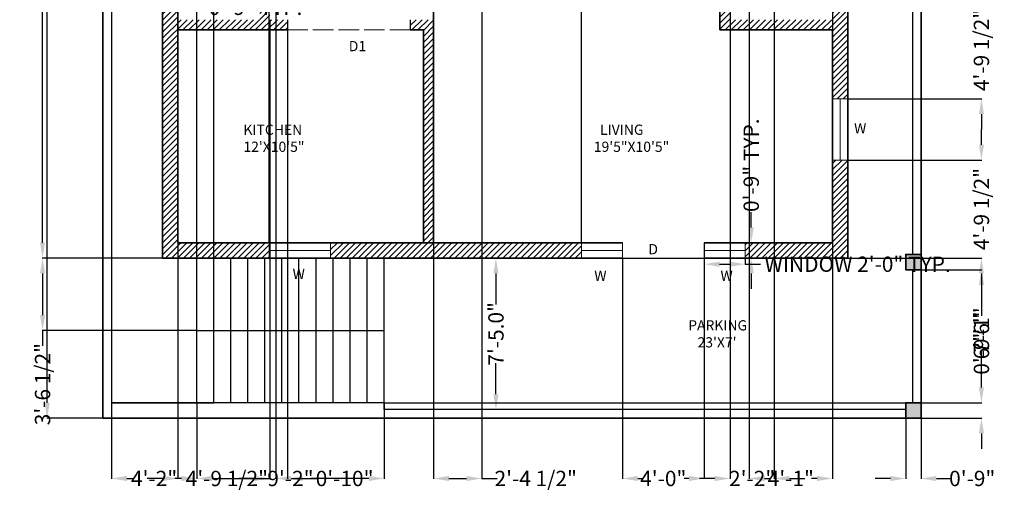
# Model space of a CAD drawing. Units: inches. Extents: x 287 to 864, y 208 to 990.
# Tile 1 of 3: x 287 to 864, y 208 to 491. Entities that reach past the tile are written whole.
import ezdxf

# ---------------------------------------------------------------- set-up
doc = ezdxf.new("R2010")
doc.units = ezdxf.units.IN
doc.header["$MEASUREMENT"] = 0
doc.linetypes.add('ACAD_ISO02W100', pattern=[15, 12, -3])
for name, color, linetype, lineweight in [('A-ANNO-DIMS', 2, 'Continuous', 18), ('A-ANNO-TEXT', 7, 'Continuous', 18), ('A-AREA-IDEN', 7, 'Continuous', 18), ('A-COLS', 7, 'Continuous', 35), ('A-DOOR', 3, 'Continuous', 25), ('A-FLOR-STRS', 7, 'Continuous', 25), ('A-GLAZ', 4, 'Continuous', 18), ('A-SITE-WALL', 7, 'Continuous', 30), ('A-WALL', 7, 'Continuous', 35), ('A-WALL-OVHD', 7, 'ACAD_ISO02W100', 18), ('C-PROP', 7, 'Continuous', 35)]:
    doc.layers.add(name, color=color, linetype=linetype, lineweight=lineweight)
doc.layers.add('A-COLS-PATT', color=18, linetype='Continuous', lineweight=13, true_color=0x000000)
doc.layers.add('A-WALL-PATT', color=240, linetype='Continuous', lineweight=13, true_color=0xed1f24)
doc.styles.get("Standard").update_dxf_attribs({"font": 'arial.ttf'})
doc.dimstyles.get("Standard").update_dxf_attribs({"dimtxt": 9, "dimasz": 9, "dimexe": 0.18, "dimexo": 0.0625, "dimgap": 0.09, "dimtad": 0, "dimdec": 1, "dimzin": 0, "dimdsep": 46, "dimlunit": 3, "dimtxsty": 'Standard', "dimcen": 0.09, "dimadec": 0, "dimazin": 0, "dimtfac": 1, "dimtdec": 1, "dimtofl": 0, "dimtmove": 0, "dimatfit": 3, "dimfxl": 1, "dimtolj": 1, "dimtzin": 0, "dimarcsym": 0})

# ---------------------------------------------------------------- blocks, each defined once
blk = doc.blocks.new('*D2')
at = {"layer": 'A-ANNO-DIMS', "color": 0, "lineweight": -2, "transparency": 16777216}
for p, q in [((335.53, 941.05), (302.65, 941.05)), ((302.83, 932.05), (302.83, 606.78)), ((302.83, 266.05), (302.83, 591.33)), ((335.53, 257.05), (302.65, 257.05))]:
    blk.add_line(p, q, dxfattribs=at)
at = {"layer": 'A-ANNO-DIMS', "color": 0, "transparency": 16777216}
for points in [[(301.33, 932.05), (304.33, 932.05), (302.83, 941.05)], [(301.33, 266.05), (304.33, 266.05), (302.83, 257.05)]]:
    blk.add_solid(points, dxfattribs=at)
at = {"layer": 'Defpoints', "color": 0, "transparency": 16777216}
for p in [(335.59, 941.05), (302.83, 257.05), (335.59, 257.05)]:
    blk.add_point(p, dxfattribs=at)
at = {"layer": 'A-ANNO-DIMS', "color": 0, "transparency": 16777216, "insert": (302.83, 599.05), "char_height": 9, "attachment_point": 5, "rotation": 90}
blk.add_mtext("\\A1;57'", dxfattribs=at)
blk = doc.blocks.new('*D5')
at = {"layer": 'A-ANNO-DIMS', "color": 0, "lineweight": -2, "transparency": 16777216}
for p, q in [((566.22, 351.05), (566.34, 351.05)), ((566.16, 342.05), (566.16, 323.81)), ((566.16, 271.05), (566.16, 289.3)), ((566.22, 262.05), (566.34, 262.05))]:
    blk.add_line(p, q, dxfattribs=at)
at = {"layer": 'A-ANNO-DIMS', "color": 0, "transparency": 16777216}
for points in [[(564.66, 342.05), (567.66, 342.05), (566.16, 351.05)], [(564.66, 271.05), (567.66, 271.05), (566.16, 262.05)]]:
    blk.add_solid(points, dxfattribs=at)
at = {"layer": 'Defpoints', "color": 0, "transparency": 16777216}
for p in [(566.16, 351.05), (566.16, 262.05), (566.16, 262.05)]:
    blk.add_point(p, dxfattribs=at)
at = {"layer": 'A-ANNO-DIMS', "color": 0, "transparency": 16777216, "insert": (566.16, 306.55), "char_height": 9, "attachment_point": 5, "rotation": 90}
blk.add_mtext('\\A1;7\'-5.0"', dxfattribs=at)
blk = doc.blocks.new('WIN-36IN')
for p, q in [((0, 9), (0, 0)), ((36, 9), (36, 0)), ((0, 4.5), (36, 4.5))]:
    blk.add_line(p, q)
blk = doc.blocks.new('WIN-24IN')
for p, q in [((0, 0), (0, 9)), ((24, 0), (24, 9)), ((24, 4.5), (0, 4.5))]:
    blk.add_line(p, q)
blk = doc.blocks.new('*D20')
at = {"layer": 'A-ANNO-DIMS', "color": 0, "lineweight": -2, "transparency": 16777216}
for p, q in [((361.59, 498.3), (352.59, 498.3)), ((370.59, 501.84), (370.59, 498.12)), ((379.59, 501.84), (379.59, 498.12)), ((388.59, 498.3), (397.59, 498.3))]:
    blk.add_line(p, q, dxfattribs=at)
at = {"layer": 'A-ANNO-DIMS', "color": 0, "transparency": 16777216}
for points in [[(361.59, 499.8), (361.59, 496.8), (370.59, 498.3)], [(388.59, 499.8), (388.59, 496.8), (379.59, 498.3)]]:
    blk.add_solid(points, dxfattribs=at)
at = {"layer": 'Defpoints', "color": 0, "transparency": 16777216}
for p in [(370.59, 501.9), (379.59, 501.9), (379.59, 498.3)]:
    blk.add_point(p, dxfattribs=at)
at = {"layer": 'A-ANNO-DIMS', "color": 0, "transparency": 16777216, "insert": (425.11, 498.3), "char_height": 9, "attachment_point": 5}
blk.add_mtext('\\A1;0\'-9" TYP.', dxfattribs=at)
blk = doc.blocks.new('*D21')
at = {"layer": 'A-ANNO-DIMS', "color": 0, "lineweight": -2, "transparency": 16777216}
for p, q in [((688.36, 350.99), (688.36, 347.27)), ((697.36, 347.45), (703.36, 347.45)), ((712.36, 350.99), (712.36, 347.27)), ((712.36, 347.45), (721.36, 347.45))]:
    blk.add_line(p, q, dxfattribs=at)
at = {"layer": 'A-ANNO-DIMS', "color": 0, "transparency": 16777216}
for points in [[(697.36, 348.95), (697.36, 345.95), (688.36, 347.45)], [(703.36, 348.95), (703.36, 345.95), (712.36, 347.45)]]:
    blk.add_solid(points, dxfattribs=at)
at = {"layer": 'Defpoints', "color": 0, "transparency": 16777216}
for p in [(688.36, 351.05), (712.36, 351.05), (712.36, 347.45)]:
    blk.add_point(p, dxfattribs=at)
at = {"layer": 'A-ANNO-DIMS', "color": 0, "transparency": 16777216, "insert": (778.39, 347.45), "char_height": 9, "attachment_point": 5}
blk.add_mtext('\\A1;WINDOW 2\'-0" TYP.', dxfattribs=at)
blk = doc.blocks.new('*D22')
at = {"layer": 'A-ANNO-DIMS', "color": 0, "lineweight": -2, "transparency": 16777216}
for p, q in [((715.96, 369.05), (715.96, 378.05)), ((712.42, 360.05), (716.14, 360.05)), ((712.42, 351.05), (716.14, 351.05)), ((715.96, 342.05), (715.96, 333.05))]:
    blk.add_line(p, q, dxfattribs=at)
at = {"layer": 'A-ANNO-DIMS', "color": 0, "transparency": 16777216}
for points in [[(714.46, 369.05), (717.46, 369.05), (715.96, 360.05)], [(714.46, 342.05), (717.46, 342.05), (715.96, 351.05)]]:
    blk.add_solid(points, dxfattribs=at)
at = {"layer": 'Defpoints', "color": 0, "transparency": 16777216}
for p in [(712.36, 360.05), (715.96, 360.05), (712.36, 351.05)]:
    blk.add_point(p, dxfattribs=at)
at = {"layer": 'A-ANNO-DIMS', "color": 0, "transparency": 16777216, "insert": (715.96, 405.57), "char_height": 9, "attachment_point": 5, "rotation": 90}
blk.add_mtext('\\A1;0\'-9" TYP.', dxfattribs=at)
blk = doc.blocks.new('*D24')
at = {"layer": 'A-ANNO-DIMS', "color": 0, "lineweight": -2, "transparency": 16777216}
for p, q in [((370.53, 906.05), (299.96, 906.05)), ((300.14, 897.05), (300.14, 644.28)), ((300.14, 360.05), (300.14, 612.83)), ((370.53, 351.05), (299.96, 351.05))]:
    blk.add_line(p, q, dxfattribs=at)
at = {"layer": 'A-ANNO-DIMS', "color": 0, "transparency": 16777216}
for points in [[(298.64, 897.05), (301.64, 897.05), (300.14, 906.05)], [(298.64, 360.05), (301.64, 360.05), (300.14, 351.05)]]:
    blk.add_solid(points, dxfattribs=at)
at = {"layer": 'Defpoints', "color": 0, "transparency": 16777216}
for p in [(300.14, 906.05), (370.59, 906.05), (370.59, 351.05)]:
    blk.add_point(p, dxfattribs=at)
at = {"layer": 'A-ANNO-DIMS', "color": 0, "transparency": 16777216, "insert": (300.14, 628.55), "char_height": 9, "attachment_point": 5, "rotation": 90}
blk.add_mtext('\\A1;46\'-3"', dxfattribs=at)
blk = doc.blocks.new('*D25')
at = {"layer": 'A-ANNO-DIMS', "color": 0, "lineweight": -2, "transparency": 16777216}
for p, q in [((390.59, 265.99), (390.59, 221.42)), ((500.59, 265.99), (500.59, 221.42)), ((399.59, 221.6), (433.54, 221.6)), ((491.59, 221.6), (457.64, 221.6))]:
    blk.add_line(p, q, dxfattribs=at)
at = {"layer": 'A-ANNO-DIMS', "color": 0, "transparency": 16777216}
for points in [[(399.59, 223.1), (399.59, 220.1), (390.59, 221.6)], [(491.59, 223.1), (491.59, 220.1), (500.59, 221.6)]]:
    blk.add_solid(points, dxfattribs=at)
at = {"layer": 'Defpoints', "color": 0, "transparency": 16777216}
for p in [(390.59, 266.05), (500.59, 266.05), (500.59, 221.6)]:
    blk.add_point(p, dxfattribs=at)
at = {"layer": 'A-ANNO-DIMS', "color": 0, "transparency": 16777216, "insert": (445.59, 221.6), "char_height": 9, "attachment_point": 5}
blk.add_mtext('\\A1;9\'-2"', dxfattribs=at)
blk = doc.blocks.new('*D26')
at = {"layer": 'A-ANNO-DIMS', "color": 0, "lineweight": -2, "transparency": 16777216}
for p, q in [((390.53, 351.05), (299.96, 351.05)), ((300.14, 342.05), (300.14, 317.55)), ((390.53, 308.55), (299.96, 308.55)), ((300.14, 308.55), (300.14, 299.55))]:
    blk.add_line(p, q, dxfattribs=at)
at = {"layer": 'A-ANNO-DIMS', "color": 0, "transparency": 16777216}
for points in [[(298.64, 342.05), (301.64, 342.05), (300.14, 351.05)], [(298.64, 317.55), (301.64, 317.55), (300.14, 308.55)]]:
    blk.add_solid(points, dxfattribs=at)
at = {"layer": 'Defpoints', "color": 0, "transparency": 16777216}
for p in [(390.59, 351.05), (300.14, 308.55), (390.59, 308.55)]:
    blk.add_point(p, dxfattribs=at)
at = {"layer": 'A-ANNO-DIMS', "color": 0, "transparency": 16777216, "insert": (300.14, 277.02), "char_height": 9, "attachment_point": 5, "rotation": 90}
blk.add_mtext('\\A1;3\'-6 1/2"', dxfattribs=at)
blk = doc.blocks.new('*D27')
at = {"layer": 'A-ANNO-DIMS', "color": 0, "lineweight": -2, "transparency": 16777216}
for p, q in [((500.65, 351.05), (851.22, 351.05)), ((851.04, 342.05), (851.04, 320.57)), ((851.04, 275.05), (851.04, 296.54)), ((500.65, 266.05), (851.22, 266.05))]:
    blk.add_line(p, q, dxfattribs=at)
at = {"layer": 'A-ANNO-DIMS', "color": 0, "transparency": 16777216}
for points in [[(849.54, 342.05), (852.54, 342.05), (851.04, 351.05)], [(849.54, 275.05), (852.54, 275.05), (851.04, 266.05)]]:
    blk.add_solid(points, dxfattribs=at)
at = {"layer": 'Defpoints', "color": 0, "transparency": 16777216}
for p in [(500.59, 351.05), (500.59, 266.05), (851.04, 266.05)]:
    blk.add_point(p, dxfattribs=at)
at = {"layer": 'A-ANNO-DIMS', "color": 0, "transparency": 16777216, "insert": (851.04, 308.55), "char_height": 9, "attachment_point": 5, "rotation": 90}
blk.add_mtext('\\A1;7\'-1"', dxfattribs=at)
blk = doc.blocks.new('*D28')
at = {"layer": 'A-ANNO-DIMS', "color": 0, "lineweight": -2, "transparency": 16777216}
for p, q in [((381.59, 976.5), (372.59, 976.5)), ((390.59, 351.12), (390.59, 976.68)), ((400.59, 351.12), (400.59, 976.68)), ((409.59, 976.5), (418.59, 976.5))]:
    blk.add_line(p, q, dxfattribs=at)
at = {"layer": 'A-ANNO-DIMS', "color": 0, "transparency": 16777216}
for points in [[(381.59, 978), (381.59, 975), (390.59, 976.5)], [(409.59, 978), (409.59, 975), (400.59, 976.5)]]:
    blk.add_solid(points, dxfattribs=at)
at = {"layer": 'Defpoints', "color": 0, "transparency": 16777216}
for p in [(400.59, 976.5), (390.59, 351.05), (400.59, 351.05)]:
    blk.add_point(p, dxfattribs=at)
at = {"layer": 'A-ANNO-DIMS', "color": 0, "transparency": 16777216, "insert": (434.14, 976.5), "char_height": 9, "attachment_point": 5}
blk.add_mtext('\\A1;0\'-10"', dxfattribs=at)
blk = doc.blocks.new('*D29')
at = {"layer": 'A-ANNO-DIMS', "color": 0, "lineweight": -2, "transparency": 16777216}
for p, q in [((340.59, 265.99), (340.59, 221.42)), ((390.59, 265.99), (390.59, 221.42)), ((349.59, 221.6), (353.36, 221.6)), ((381.59, 221.6), (377.82, 221.6))]:
    blk.add_line(p, q, dxfattribs=at)
at = {"layer": 'A-ANNO-DIMS', "color": 0, "transparency": 16777216}
for points in [[(349.59, 223.1), (349.59, 220.1), (340.59, 221.6)], [(381.59, 223.1), (381.59, 220.1), (390.59, 221.6)]]:
    blk.add_solid(points, dxfattribs=at)
at = {"layer": 'Defpoints', "color": 0, "transparency": 16777216}
for p in [(340.59, 266.05), (390.59, 266.05), (390.59, 221.6)]:
    blk.add_point(p, dxfattribs=at)
at = {"layer": 'A-ANNO-DIMS', "color": 0, "transparency": 16777216, "insert": (365.59, 221.6), "char_height": 9, "attachment_point": 5}
blk.add_mtext('\\A1;4\'-2"', dxfattribs=at)
blk = doc.blocks.new('*D30')
at = {"layer": 'A-ANNO-DIMS', "color": 0, "lineweight": -2, "transparency": 16777216}
for p, q in [((640.36, 350.99), (640.36, 221.42)), ((688.36, 350.99), (688.36, 221.42)), ((649.36, 221.6), (652.13, 221.6)), ((679.36, 221.6), (676.59, 221.6))]:
    blk.add_line(p, q, dxfattribs=at)
at = {"layer": 'A-ANNO-DIMS', "color": 0, "transparency": 16777216}
for points in [[(649.36, 223.1), (649.36, 220.1), (640.36, 221.6)], [(679.36, 223.1), (679.36, 220.1), (688.36, 221.6)]]:
    blk.add_solid(points, dxfattribs=at)
at = {"layer": 'Defpoints', "color": 0, "transparency": 16777216}
for p in [(640.36, 351.05), (688.36, 351.05), (688.36, 221.6)]:
    blk.add_point(p, dxfattribs=at)
at = {"layer": 'A-ANNO-DIMS', "color": 0, "transparency": 16777216, "insert": (664.36, 221.6), "char_height": 9, "attachment_point": 5}
blk.add_mtext('\\A1;4\'-0"', dxfattribs=at)
blk = doc.blocks.new('*D32')
at = {"layer": 'A-ANNO-DIMS', "color": 0, "lineweight": -2, "transparency": 16777216}
for p, q in [((433.59, 490.99), (433.59, 221.42)), ((443.82, 484.99), (443.82, 221.42)), ((424.59, 221.6), (415.59, 221.6)), ((452.82, 221.6), (461.82, 221.6))]:
    blk.add_line(p, q, dxfattribs=at)
at = {"layer": 'A-ANNO-DIMS', "color": 0, "transparency": 16777216}
for points in [[(424.59, 223.1), (424.59, 220.1), (433.59, 221.6)], [(452.82, 223.1), (452.82, 220.1), (443.82, 221.6)]]:
    blk.add_solid(points, dxfattribs=at)
at = {"layer": 'Defpoints', "color": 0, "transparency": 16777216}
for p in [(433.59, 491.05), (443.82, 485.05), (443.82, 221.6)]:
    blk.add_point(p, dxfattribs=at)
at = {"layer": 'A-ANNO-DIMS', "color": 0, "transparency": 16777216, "insert": (477.37, 221.6), "char_height": 9, "attachment_point": 5}
blk.add_mtext('\\A1;0\'-10"', dxfattribs=at)
blk = doc.blocks.new('*D33')
at = {"layer": 'A-ANNO-DIMS', "color": 0, "lineweight": -2, "transparency": 16777216}
for p, q in [((379.59, 896.99), (379.59, 221.42)), ((436.99, 896.99), (436.99, 221.42)), ((370.59, 221.6), (361.59, 221.6)), ((445.99, 221.6), (454.99, 221.6))]:
    blk.add_line(p, q, dxfattribs=at)
at = {"layer": 'A-ANNO-DIMS', "color": 0, "transparency": 16777216}
for points in [[(370.59, 223.1), (370.59, 220.1), (379.59, 221.6)], [(445.99, 223.1), (445.99, 220.1), (436.99, 221.6)]]:
    blk.add_solid(points, dxfattribs=at)
at = {"layer": 'Defpoints', "color": 0, "transparency": 16777216}
for p in [(379.59, 897.05), (436.99, 897.05), (436.99, 221.6)]:
    blk.add_point(p, dxfattribs=at)
at = {"layer": 'A-ANNO-DIMS', "color": 0, "transparency": 16777216, "insert": (408.29, 221.6), "char_height": 9, "attachment_point": 5}
blk.add_mtext('\\A1;4\'-9 1/2"', dxfattribs=at)
blk = doc.blocks.new('*D34')
at = {"layer": 'A-ANNO-DIMS', "color": 0, "lineweight": -2, "transparency": 16777216}
for p, q in [((529.59, 896.99), (529.59, 221.42)), ((557.92, 896.99), (557.92, 221.42)), ((538.59, 221.6), (548.92, 221.6)), ((557.92, 221.6), (566.92, 221.6))]:
    blk.add_line(p, q, dxfattribs=at)
at = {"layer": 'A-ANNO-DIMS', "color": 0, "transparency": 16777216}
for points in [[(538.59, 223.1), (538.59, 220.1), (529.59, 221.6)], [(548.92, 223.1), (548.92, 220.1), (557.92, 221.6)]]:
    blk.add_solid(points, dxfattribs=at)
at = {"layer": 'Defpoints', "color": 0, "transparency": 16777216}
for p in [(529.59, 897.05), (557.92, 897.05), (557.92, 221.6)]:
    blk.add_point(p, dxfattribs=at)
at = {"layer": 'A-ANNO-DIMS', "color": 0, "transparency": 16777216, "insert": (589.53, 221.6), "char_height": 9, "attachment_point": 5}
blk.add_mtext('\\A1;2\'-4 1/2"', dxfattribs=at)
blk = doc.blocks.new('*D35')
at = {"layer": 'A-ANNO-DIMS', "color": 0, "lineweight": -2, "transparency": 16777216}
for p, q in [((714.78, 896.99), (714.78, 221.42)), ((763.59, 896.99), (763.59, 221.42)), ((723.78, 221.6), (726.95, 221.6)), ((754.59, 221.6), (751.42, 221.6))]:
    blk.add_line(p, q, dxfattribs=at)
at = {"layer": 'A-ANNO-DIMS', "color": 0, "transparency": 16777216}
for points in [[(723.78, 223.1), (723.78, 220.1), (714.78, 221.6)], [(754.59, 223.1), (754.59, 220.1), (763.59, 221.6)]]:
    blk.add_solid(points, dxfattribs=at)
at = {"layer": 'Defpoints', "color": 0, "transparency": 16777216}
for p in [(714.78, 897.05), (763.59, 897.05), (763.59, 221.6)]:
    blk.add_point(p, dxfattribs=at)
at = {"layer": 'A-ANNO-DIMS', "color": 0, "transparency": 16777216, "insert": (739.19, 221.6), "char_height": 9, "attachment_point": 5}
blk.add_mtext('\\A1;4\'-1"', dxfattribs=at)
blk = doc.blocks.new('*D37')
at = {"layer": 'A-ANNO-DIMS', "color": 0, "lineweight": -2, "transparency": 16777216}
for p, q in [((851.04, 510.9), (851.04, 519.9)), ((772.65, 501.9), (851.22, 501.9)), ((772.65, 444.61), (851.22, 444.61)), ((851.04, 435.61), (851.04, 426.61))]:
    blk.add_line(p, q, dxfattribs=at)
at = {"layer": 'A-ANNO-DIMS', "color": 0, "transparency": 16777216}
for points in [[(849.54, 510.9), (852.54, 510.9), (851.04, 501.9)], [(849.54, 435.61), (852.54, 435.61), (851.04, 444.61)]]:
    blk.add_solid(points, dxfattribs=at)
at = {"layer": 'Defpoints', "color": 0, "transparency": 16777216}
for p in [(772.59, 501.9), (851.04, 501.9), (772.59, 444.61)]:
    blk.add_point(p, dxfattribs=at)
at = {"layer": 'A-ANNO-DIMS', "color": 0, "transparency": 16777216, "insert": (851.04, 473.26), "char_height": 9, "attachment_point": 5, "rotation": 90}
blk.add_mtext('\\A1;4\'-9 1/2"', dxfattribs=at)
blk = doc.blocks.new('*D38')
at = {"layer": 'A-ANNO-DIMS', "color": 0, "lineweight": -2, "transparency": 16777216}
for p, q in [((851.04, 417.61), (851.04, 426.61)), ((772.65, 408.61), (851.22, 408.61)), ((772.65, 351.05), (851.22, 351.05)), ((851.04, 342.05), (851.04, 333.05))]:
    blk.add_line(p, q, dxfattribs=at)
at = {"layer": 'A-ANNO-DIMS', "color": 0, "transparency": 16777216}
for points in [[(849.54, 417.61), (852.54, 417.61), (851.04, 408.61)], [(849.54, 342.05), (852.54, 342.05), (851.04, 351.05)]]:
    blk.add_solid(points, dxfattribs=at)
at = {"layer": 'Defpoints', "color": 0, "transparency": 16777216}
for p in [(772.59, 408.61), (851.04, 408.61), (772.59, 351.05)]:
    blk.add_point(p, dxfattribs=at)
at = {"layer": 'A-ANNO-DIMS', "color": 0, "transparency": 16777216, "insert": (851.04, 379.83), "char_height": 9, "attachment_point": 5, "rotation": 90}
blk.add_mtext('\\A1;4\'-9 1/2"', dxfattribs=at)
blk = doc.blocks.new('*D39')
at = {"layer": 'A-ANNO-DIMS', "color": 0, "lineweight": -2, "transparency": 16777216}
for p, q in [((370.59, 976.5), (361.59, 976.5)), ((379.59, 360.12), (379.59, 976.68)), ((433.14, 360.12), (433.14, 976.68)), ((442.14, 976.5), (451.14, 976.5))]:
    blk.add_line(p, q, dxfattribs=at)
at = {"layer": 'A-ANNO-DIMS', "color": 0, "transparency": 16777216}
for points in [[(370.59, 978), (370.59, 975), (379.59, 976.5)], [(442.14, 978), (442.14, 975), (433.14, 976.5)]]:
    blk.add_solid(points, dxfattribs=at)
at = {"layer": 'Defpoints', "color": 0, "transparency": 16777216}
for p in [(433.14, 976.5), (379.59, 360.05), (433.14, 360.05)]:
    blk.add_point(p, dxfattribs=at)
at = {"layer": 'A-ANNO-DIMS', "color": 0, "transparency": 16777216, "insert": (406.37, 976.5), "char_height": 9, "attachment_point": 5}
blk.add_mtext('\\A1;4\'-5 1/2"', dxfattribs=at)
blk = doc.blocks.new('*D40')
at = {"layer": 'A-ANNO-DIMS', "color": 0, "lineweight": -2, "transparency": 16777216}
for p, q in [((529.59, 360.12), (529.59, 976.68)), ((538.59, 976.5), (560.96, 976.5)), ((607.36, 976.5), (584.99, 976.5)), ((616.36, 360.12), (616.36, 976.68))]:
    blk.add_line(p, q, dxfattribs=at)
at = {"layer": 'A-ANNO-DIMS', "color": 0, "transparency": 16777216}
for points in [[(538.59, 978), (538.59, 975), (529.59, 976.5)], [(607.36, 978), (607.36, 975), (616.36, 976.5)]]:
    blk.add_solid(points, dxfattribs=at)
at = {"layer": 'Defpoints', "color": 0, "transparency": 16777216}
for p in [(616.36, 976.5), (529.59, 360.05), (616.36, 360.05)]:
    blk.add_point(p, dxfattribs=at)
at = {"layer": 'A-ANNO-DIMS', "color": 0, "transparency": 16777216, "insert": (572.97, 976.5), "char_height": 9, "attachment_point": 5}
blk.add_mtext('\\A1;7\'-3"', dxfattribs=at)
blk = doc.blocks.new('*D47')
at = {"layer": 'A-ANNO-DIMS', "color": 0, "lineweight": -2, "transparency": 16777216}
for p, q in [((703.59, 584.99), (703.59, 221.42)), ((729.41, 584.99), (729.41, 221.42)), ((694.59, 221.6), (685.59, 221.6)), ((738.41, 221.6), (747.41, 221.6))]:
    blk.add_line(p, q, dxfattribs=at)
at = {"layer": 'A-ANNO-DIMS', "color": 0, "transparency": 16777216}
for points in [[(694.59, 223.1), (694.59, 220.1), (703.59, 221.6)], [(738.41, 223.1), (738.41, 220.1), (729.41, 221.6)]]:
    blk.add_solid(points, dxfattribs=at)
at = {"layer": 'Defpoints', "color": 0, "transparency": 16777216}
for p in [(703.59, 585.05), (729.41, 585.05), (729.41, 221.6)]:
    blk.add_point(p, dxfattribs=at)
at = {"layer": 'A-ANNO-DIMS', "color": 0, "transparency": 16777216, "insert": (716.5, 221.6), "char_height": 9, "attachment_point": 5}
blk.add_mtext('\\A1;2\'-2"', dxfattribs=at)
blk = doc.blocks.new('*D48')
at = {"layer": 'A-ANNO-DIMS', "color": 0, "lineweight": -2, "transparency": 16777216}
for p, q in [((815.65, 344.19), (851.22, 344.19)), ((851.04, 335.19), (851.04, 317.2)), ((851.04, 275.05), (851.04, 293.04)), ((815.65, 266.05), (851.22, 266.05))]:
    blk.add_line(p, q, dxfattribs=at)
at = {"layer": 'A-ANNO-DIMS', "color": 0, "transparency": 16777216}
for points in [[(849.54, 335.19), (852.54, 335.19), (851.04, 344.19)], [(849.54, 275.05), (852.54, 275.05), (851.04, 266.05)]]:
    blk.add_solid(points, dxfattribs=at)
at = {"layer": 'Defpoints', "color": 0, "transparency": 16777216}
for p in [(815.59, 344.19), (851.04, 344.19), (815.59, 266.05)]:
    blk.add_point(p, dxfattribs=at)
at = {"layer": 'A-ANNO-DIMS', "color": 0, "transparency": 16777216, "insert": (851.04, 305.12), "char_height": 9, "attachment_point": 5, "rotation": 90}
blk.add_mtext('\\A1;6\'-6"', dxfattribs=at)
blk = doc.blocks.new('*D49')
at = {"layer": 'A-ANNO-DIMS', "color": 0, "lineweight": -2, "transparency": 16777216}
for p, q in [((806.59, 256.99), (806.59, 221.42)), ((815.59, 256.99), (815.59, 221.42)), ((797.59, 221.6), (788.59, 221.6)), ((824.59, 221.6), (833.59, 221.6))]:
    blk.add_line(p, q, dxfattribs=at)
at = {"layer": 'A-ANNO-DIMS', "color": 0, "transparency": 16777216}
for points in [[(797.59, 223.1), (797.59, 220.1), (806.59, 221.6)], [(824.59, 223.1), (824.59, 220.1), (815.59, 221.6)]]:
    blk.add_solid(points, dxfattribs=at)
at = {"layer": 'Defpoints', "color": 0, "transparency": 16777216}
for p in [(806.59, 257.05), (815.59, 257.05), (815.59, 221.6)]:
    blk.add_point(p, dxfattribs=at)
at = {"layer": 'A-ANNO-DIMS', "color": 0, "transparency": 16777216, "insert": (845.64, 221.6), "char_height": 9, "attachment_point": 5}
blk.add_mtext('\\A1;0\'-9"', dxfattribs=at)
blk = doc.blocks.new('*D50')
at = {"layer": 'A-ANNO-DIMS', "color": 0, "lineweight": -2, "transparency": 16777216}
for p, q in [((851.04, 275.05), (851.04, 284.05)), ((815.65, 266.05), (851.22, 266.05)), ((815.65, 257.05), (851.22, 257.05)), ((851.04, 248.05), (851.04, 239.05))]:
    blk.add_line(p, q, dxfattribs=at)
at = {"layer": 'A-ANNO-DIMS', "color": 0, "transparency": 16777216}
for points in [[(849.54, 275.05), (852.54, 275.05), (851.04, 266.05)], [(849.54, 248.05), (852.54, 248.05), (851.04, 257.05)]]:
    blk.add_solid(points, dxfattribs=at)
at = {"layer": 'Defpoints', "color": 0, "transparency": 16777216}
for p in [(815.59, 266.05), (851.04, 266.05), (815.59, 257.05)]:
    blk.add_point(p, dxfattribs=at)
at = {"layer": 'A-ANNO-DIMS', "color": 0, "transparency": 16777216, "insert": (851.04, 296.11), "char_height": 9, "attachment_point": 5, "rotation": 90}
blk.add_mtext('\\A1;0\'-9"', dxfattribs=at)

msp = doc.modelspace()

# ---------------------------------------------------------------- hatches: boundary and pattern name
at = {"layer": 'A-COLS-PATT'}
h = msp.add_hatch(color=256, dxfattribs=at)
h.dxf.hatch_style = 1
h.paths.add_polyline_path([(815.59, 353.19), (806.59, 353.19), (806.59, 344.19), (815.59, 344.19)])
h.paths.add_polyline_path([(815.59, 266.05), (806.59, 266.05), (806.59, 257.05), (815.59, 257.05)])
at = {"layer": 'A-WALL-PATT'}
h = msp.add_hatch(dxfattribs=at)
h.set_pattern_fill('ANSI31', color=256, scale=20)
h.paths.add_polyline_path([(443.82, 491.05), (433.59, 491.05), (433.59, 585.05), (529.59, 585.05), (529.59, 690.13), (523.59, 690.13), (523.59, 591.05), (420.92, 591.05), (420.92, 585.05), (427.59, 585.05), (427.59, 491.05), (379.59, 491.05), (379.59, 501.9), (370.59, 501.9), (370.59, 351.05), (433.14, 351.05), (433.14, 360.05), (379.59, 360.05), (379.59, 485.05), (443.82, 485.05)])
h.paths.add_polyline_path([(616.36, 360.05), (469.14, 360.05), (469.14, 351.05), (616.36, 351.05)])
h.paths.add_polyline_path([(772.59, 647.65), (763.59, 647.65), (763.59, 591.05), (753.41, 591.05), (753.41, 585.05), (763.59, 585.05), (763.59, 525.9), (772.59, 525.9)])
h.paths.add_polyline_path([(772.59, 906.05), (714.78, 906.05), (714.78, 897.05), (763.59, 897.05), (763.59, 741.05), (619.59, 741.05), (619.59, 749.52), (613.59, 749.52), (613.59, 637.13), (619.59, 637.13), (619.59, 735.05), (763.59, 735.05), (763.59, 683.65), (772.59, 683.65)])
h.paths.add_polyline_path([(678.78, 906.05), (581.92, 906.05), (581.92, 897.05), (613.59, 897.05), (613.59, 849.05), (529.59, 849.05), (529.59, 854.59), (523.59, 854.59), (523.59, 785.52), (529.59, 785.52), (529.59, 789.05), (613.59, 789.05), (613.59, 785.52), (619.59, 785.52), (619.59, 812.74), (613.59, 812.74), (613.59, 795.05), (529.59, 795.05), (529.59, 843.05), (613.59, 843.05), (613.59, 836.74), (619.59, 836.74), (619.59, 897.05), (678.78, 897.05)])
h.paths.add_polyline_path([(557.92, 906.05), (472.99, 906.05), (472.99, 897.05), (523.59, 897.05), (523.59, 878.59), (529.59, 878.59), (529.59, 897.05), (557.92, 897.05)])
h.paths.add_polyline_path([(436.99, 906.05), (370.59, 906.05), (370.59, 683.65), (379.59, 683.65), (379.59, 735.05), (523.59, 735.05), (523.59, 726.13), (529.59, 726.13), (529.59, 749.52), (523.59, 749.52), (523.59, 741.05), (379.59, 741.05), (379.59, 897.05), (436.99, 897.05)])
h.paths.add_polyline_path([(379.59, 647.65), (370.59, 647.65), (370.59, 525.9), (379.59, 525.9), (379.59, 585.05), (396.92, 585.05), (396.92, 591.05), (379.59, 591.05)], flags=17)
h.paths.add_polyline_path([(529.59, 491.05), (515.82, 491.05), (515.82, 485.05), (523.59, 485.05), (523.59, 360.05), (529.59, 360.05)], flags=17)
h.paths.add_polyline_path([(763.59, 444.61), (772.59, 444.61), (772.59, 501.9), (763.59, 501.9), (763.59, 491.05), (703.59, 491.05), (703.59, 585.05), (729.41, 585.05), (729.41, 591.05), (619.59, 591.05), (619.59, 601.13), (613.59, 601.13), (613.59, 585.05), (697.59, 585.05), (697.59, 485.05), (763.59, 485.05)])
h.paths.add_polyline_path([(772.59, 408.61), (763.59, 408.61), (763.59, 360.05), (712.36, 360.05), (712.36, 351.05), (772.59, 351.05)])

# ---------------------------------------------------------------- linework, layer by layer
at = {"layer": 'A-COLS'}
for points in [[(815.59, 344.19), (806.59, 344.19), (806.59, 353.19), (815.59, 353.19)], [(815.59, 257.05), (806.59, 257.05), (806.59, 266.05), (815.59, 266.05)]]:
    msp.add_lwpolyline(points, close=True, dxfattribs=at)
at = {"layer": 'A-DOOR'}
for p, q in [((443.82, 491.05), (443.82, 485.05)), ((515.82, 491.05), (515.82, 485.05)), ((688.36, 360.05), (688.36, 351.05))]:
    msp.add_line(p, q, dxfattribs=at)
at = {"layer": 'A-FLOR-STRS'}
for p, q in [((370.59, 351.05), (340.59, 351.05)), ((390.59, 266.05), (390.59, 351.05)), ((400.59, 266.05), (400.59, 351.05)), ((410.59, 266.05), (410.59, 351.05)), ((420.59, 266.05), (420.59, 351.05)), ((430.59, 266.05), (430.59, 351.05)), ((440.59, 266.05), (440.59, 351.05)), ((450.59, 266.05), (450.59, 351.05)), ((460.59, 266.05), (460.59, 351.05)), ((470.59, 266.05), (470.59, 351.05)), ((480.59, 266.05), (480.59, 351.05)), ((490.59, 266.05), (490.59, 351.05)), ((500.59, 262.05), (500.59, 351.05)), ((390.59, 308.55), (500.59, 308.55)), ((500.59, 266.05), (340.59, 266.05)), ((340.59, 266.05), (376.59, 266.05)), ((376.59, 266.05), (400.59, 266.05))]:
    msp.add_line(p, q, dxfattribs=at)
at = {"layer": 'A-GLAZ'}
msp.add_line((616.36, 351.05), (616.36, 360.05), dxfattribs=at)
at = {"layer": 'A-SITE-WALL'}
for p, q in [((340.59, 936.05), (340.59, 266.05)), ((810.59, 936.05), (810.59, 353.19)), ((810.59, 344.19), (810.59, 266.05)), ((806.59, 262.05), (500.59, 262.05))]:
    msp.add_line(p, q, dxfattribs=at)
at = {"layer": 'A-WALL'}
for p, q in [((370.59, 351.05), (370.59, 906.05)), ((772.59, 906.05), (772.59, 351.05)), ((697.59, 585.05), (697.59, 485.05)), ((529.59, 360.05), (529.59, 491.05)), ((379.59, 360.05), (379.59, 485.05)), ((443.82, 485.05), (379.59, 485.05)), ((523.59, 485.05), (515.82, 485.05)), ((523.59, 360.05), (523.59, 485.05)), ((763.59, 485.05), (697.59, 485.05)), ((763.59, 485.05), (763.59, 360.05)), ((640.36, 360.05), (379.59, 360.05)), ((763.59, 360.05), (688.36, 360.05)), ((640.36, 351.05), (370.59, 351.05)), ((772.59, 351.05), (688.36, 351.05))]:
    msp.add_line(p, q, dxfattribs=at)
at = {"layer": 'A-WALL-OVHD'}
msp.add_line((443.82, 485.05), (515.82, 485.05), dxfattribs=at)
at = {"layer": 'C-PROP'}
for p, q in [((335.59, 257.05), (335.59, 941.05)), ((815.59, 941.05), (815.59, 257.05)), ((815.59, 257.05), (335.59, 257.05))]:
    msp.add_line(p, q, dxfattribs=at)

# ---------------------------------------------------------------- block references
at = {"layer": 'A-GLAZ'}
for name, p, rotation in [('WIN-36IN', (763.59, 444.61), 269.9999999999999), ('WIN-24IN', (640.36, 360.05), 180)]:
    msp.add_blockref(name, p, dxfattribs=dict(at, rotation=rotation))
for name, p in [('WIN-36IN', (433.14, 351.05)), ('WIN-24IN', (688.36, 351.05))]:
    msp.add_blockref(name, p, dxfattribs=at)

# ---------------------------------------------------------------- texts
at = {"layer": 'A-ANNO-TEXT', "char_height": 6, "attachment_point": 1}
for s, insert in [('D1', (479.82, 478.53)), ('W', (776.32, 430.24)), ('D', (655.62, 359.24)), ('W', (446.87, 344.74)), ('W', (623.88, 343.64)), ('W', (697.92, 343.64))]:
    msp.add_mtext_dynamic_manual_height_columns(s, width=80.3005, gutter_width=1, heights=[0], dxfattribs=dict(at, insert=insert))
at = {"layer": 'A-AREA-IDEN', "char_height": 6, "attachment_point": 1}
for s, insert in [('KITCHEN\\P12\'X10\'5"', (417.99, 429.42)), ('  LIVING\\P19\'5"X10\'5"', (623.59, 429.42)), ("  PARKING\\P     23'X7'", (675.3, 314.56))]:
    msp.add_mtext_dynamic_manual_height_columns(s, width=80.3005, gutter_width=1, heights=[0], dxfattribs=dict(at, insert=insert))

# ---------------------------------------------------------------- dimensions: what is measured, and where the dimension line sits
at = {"layer": 'A-ANNO-DIMS'}
for base, p1, p2, picture, middle in [((433.1449, 976.5045), (379.5899, 360.0545), (433.1449, 360.0545), '*D39', (406.3674, 976.5045)), ((400.59, 976.5), (390.59, 351.05), (400.59, 351.05), '*D28', (434.14, 976.5)), ((616.36, 976.5), (529.59, 360.05), (616.36, 360.05), '*D40', (572.97, 976.5)), ((436.99, 221.6), (379.59, 897.05), (436.99, 897.05), '*D33', (408.29, 221.6)), ((557.92, 221.6), (529.59, 897.05), (557.92, 897.05), '*D34', (589.53, 221.6)), ((763.59, 221.6), (714.78, 897.05), (763.59, 897.05), '*D35', (739.19, 221.6)), ((729.41, 221.6), (703.59, 585.05), (729.41, 585.05), '*D47', (716.5, 221.6)), ((443.82, 221.6), (433.59, 491.05), (443.82, 485.05), '*D32', (477.37, 221.6)), ((688.36, 221.6), (640.36, 351.05), (688.36, 351.05), '*D30', (664.36, 221.6)), ((390.59, 221.6), (340.59, 266.05), (390.59, 266.05), '*D29', (365.59, 221.6)), ((500.59, 221.6), (390.59, 266.05), (500.59, 266.05), '*D25', (445.59, 221.6)), ((815.59, 221.6), (806.59, 257.05), (815.59, 257.05), '*D49', (845.64, 221.6))]:
    dim = msp.add_linear_dim(base=base, p1=p1, p2=p2, dimstyle='Standard', override={"dimdec": 1, "dimlfac": 1, "dimrnd": 0, "dimzin": 1, "dimdsep": 46, "dimlunit": 4, "dimfrac": 2}, dxfattribs=at)
    dim.commit()
    dim.dimension.update_dxf_attribs({"geometry": picture, "text_midpoint": middle})
for base, p1, p2, override, picture, middle in [((302.83, 257.05), (335.59, 941.05), (335.59, 257.05), {"dimclrd": 0, "dimclre": 0, "dimclrt": 0}, '*D2', (302.83, 599.05)), ((300.14, 906.05), (370.59, 351.05), (370.59, 906.05), {"dimdec": 1, "dimlfac": 1, "dimrnd": 0, "dimzin": 1, "dimdsep": 46, "dimlunit": 4, "dimfrac": 2}, '*D24', (300.14, 628.55)), ((851.04, 501.9), (772.59, 444.61), (772.59, 501.9), {"dimdec": 1, "dimlfac": 1, "dimrnd": 0, "dimzin": 1, "dimdsep": 46, "dimlunit": 4, "dimfrac": 2}, '*D37', (851.04, 473.26)), ((851.04, 408.61), (772.59, 351.05), (772.59, 408.61), {"dimdec": 1, "dimlfac": 1, "dimrnd": 0, "dimzin": 1, "dimdsep": 46, "dimlunit": 4, "dimfrac": 2}, '*D38', (851.04, 379.83)), ((300.14, 308.55), (390.59, 351.05), (390.59, 308.55), {"dimdec": 1, "dimlfac": 1, "dimrnd": 0, "dimzin": 1, "dimdsep": 46, "dimlunit": 4, "dimfrac": 2}, '*D26', (300.14, 277.02)), ((851.04, 266.05), (500.59, 351.05), (500.59, 266.05), {"dimdec": 1, "dimlfac": 1, "dimrnd": 0, "dimzin": 1, "dimdsep": 46, "dimlunit": 4, "dimfrac": 2}, '*D27', (851.04, 308.55)), ((566.16, 262.05), (566.16, 351.05), (566.16, 262.05), {"dimclrd": 0, "dimclre": 0, "dimclrt": 0}, '*D5', (566.16, 306.55)), ((851.04, 344.19), (815.59, 266.05), (815.59, 344.19), {"dimdec": 1, "dimlfac": 1, "dimrnd": 0, "dimzin": 1, "dimdsep": 46, "dimlunit": 4, "dimfrac": 2}, '*D48', (851.04, 305.12)), ((851.04, 266.05), (815.59, 257.05), (815.59, 266.05), {"dimdec": 1, "dimlfac": 1, "dimrnd": 0, "dimzin": 1, "dimdsep": 46, "dimlunit": 4, "dimfrac": 2}, '*D50', (851.04, 296.11))]:
    dim = msp.add_linear_dim(base=base, p1=p1, p2=p2, angle=90, dimstyle='Standard', override=override, dxfattribs=at)
    dim.commit()
    dim.dimension.update_dxf_attribs({"geometry": picture, "text_midpoint": middle})
for base, p1, p2, text, picture, middle in [((379.59, 498.3), (370.59, 501.9), (379.59, 501.9), '<> TYP.', '*D20', (425.11, 498.3)), ((712.36, 347.45), (688.36, 351.05), (712.36, 351.05), 'WINDOW <> TYP.', '*D21', (778.39, 347.45))]:
    dim = msp.add_linear_dim(base=base, p1=p1, p2=p2, text=text, dimstyle='Standard', override={"dimdec": 1, "dimlfac": 1, "dimrnd": 0, "dimzin": 1, "dimdsep": 46, "dimlunit": 4, "dimfrac": 2}, dxfattribs=at)
    dim.commit()
    dim.dimension.update_dxf_attribs({"geometry": picture, "text_midpoint": middle})
dim = msp.add_linear_dim(base=(715.96, 360.05), p1=(712.36, 351.05), p2=(712.36, 360.05), angle=90, text='<> TYP.', dimstyle='Standard', override={"dimdec": 1, "dimlfac": 1, "dimrnd": 0, "dimzin": 1, "dimdsep": 46, "dimlunit": 4, "dimfrac": 2}, dxfattribs=at)
dim.commit()
dim.dimension.update_dxf_attribs({"geometry": '*D22', "text_midpoint": (715.96, 405.57)})

doc.saveas('drawing.dxf')
